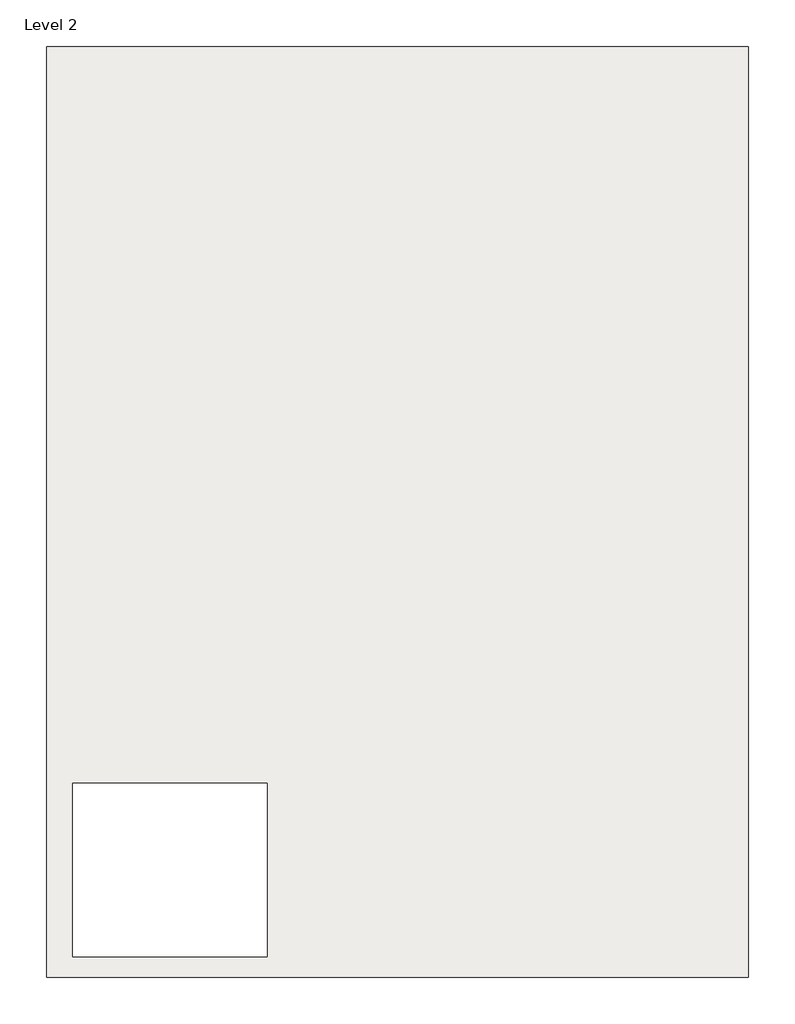
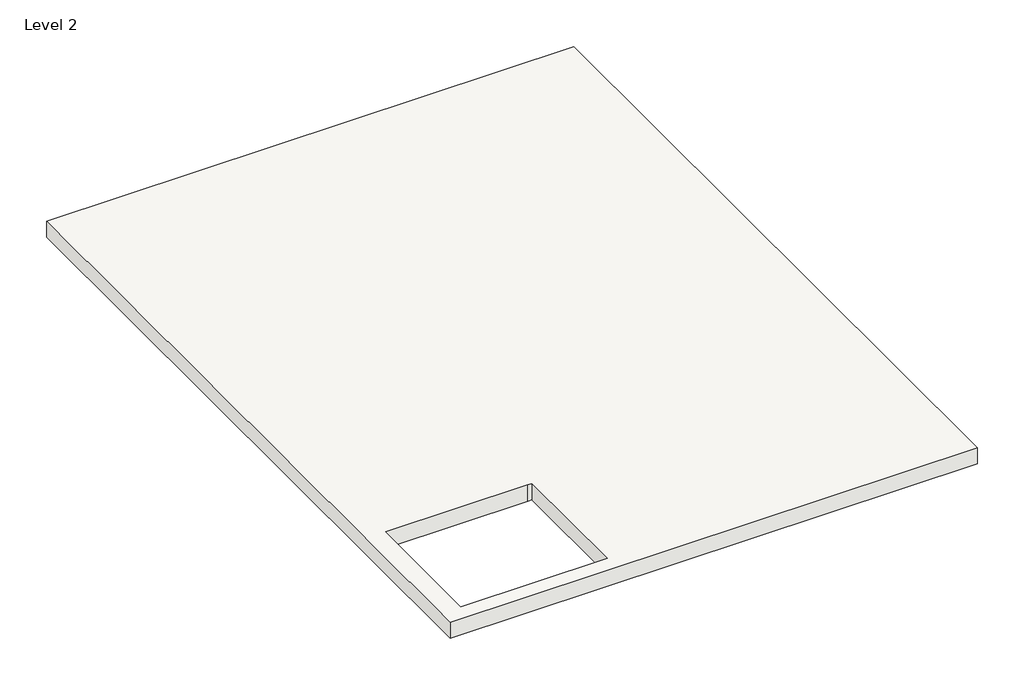
# One storey: 1 roof.
"""IFC4 building model written with IfcOpenShell, lengths in millimetres."""

from ifc_helpers import new_model, si_unit, frame, origin, place, context, project, spatial, polyline, outline, extrude, element, save

model = new_model("IFC4")

# Units and contexts
model_context = context("Model", 3, world=origin())
ifc_project = project(units=[si_unit("LENGTHUNIT", "METRE", prefix="MILLI")], contexts=[model_context])

# Site, building, storey
site = spatial("IfcSite", under=ifc_project)
building = spatial("IfcBuilding", under=site)
storey = spatial("IfcBuildingStorey", under=building, Name="Level 2", Elevation=3048.0)

# Roof
placement = place(None, origin())
element("IfcRoof", 1, ObjectType="Generic - 12\"", at=placement, inside=storey, context=model_context, shape_type="SweptSolid", body=[
    extrude(outline(polyline([(-11433.0073372, 14222.3174997), (-2085.8073372, 14222.3174997), (-2085.8073372, 1827.1174997), (-11433.0073372, 1827.1174997), (-11433.0073372, 14222.3174997)]), holes=[polyline([(-8491.8071173, 4414.3732459), (-8568.0071173, 4414.3732459), (-11082.6071173, 4414.3732459), (-11082.6071173, 2102.9732459), (-8491.8071173, 2102.9732459), (-8491.8071173, 4414.3732459)])]), frame((0.0, 0.0, 3048.0), z_axis=(0.0, 0.0, 1.0), x_axis=(1.0, 0.0, 0.0)), (0.0, 0.0, 1.0), 304.8),
])

save(model, "model.ifc")

# Revit data of these elements
# Type "Generic - 12\""
#   Assembly Code = "B1020"
#   Layers, outside or top first: 1' - 0" "Brick, Soldier Course" (function 1)
# Element 1 (IfcRoof, "Generic - 12\"")
#   built-in parameter 1001705 = 11 (stored number, unit not read)
#   built-in parameter 1001710 = 33615
#   Phase Created = New Construction
#   Materials on its faces: "Brick, Soldier Course"
# Materials
#   "Brick, Soldier Course": class "Masonry", colour RGB 170 98 104, transparency 0, Description = "Common brick soldier coursed", Cost = 0
